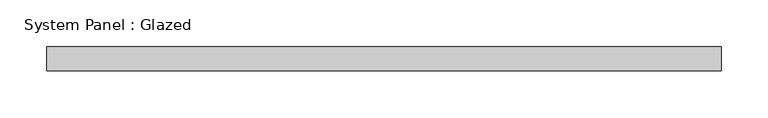
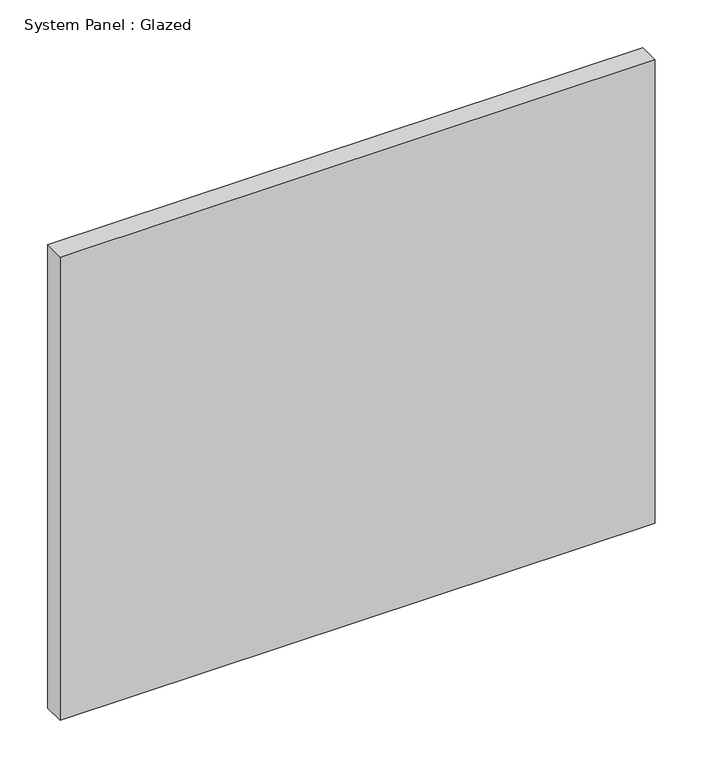
"""IFC4 building model written with IfcOpenShell, lengths in millimetres: plate geometry, System Panel : Glazed."""

from ifc_helpers import new_model, si_unit, origin, origin_with_axes, place, context, project, spatial, polyline, outline, extrude, source, transform, mapped, element, save


def system_panel_glazed_ba8d0b35(model_context):
    return source(origin(), model_context, "Body", "SweptSolid", [
        extrude(outline(polyline([(358.775, 19.05), (-358.775, 19.05), (-358.775, 44.45), (358.775, 44.45), (358.775, 19.05)])), origin_with_axes(), (0.0, 0.0, 1.0), 590.2074877),
    ])


if __name__ == "__main__":
    model = new_model("IFC4")
    model_context = context("Model", 3, world=origin())
    ifc_project = project(units=[si_unit("LENGTHUNIT", "METRE", prefix="MILLI")], contexts=[model_context])
    site = spatial("IfcSite", under=ifc_project)
    building = spatial("IfcBuilding", under=site)
    placement = place(None, origin())
    system_panel_glazed_shape = system_panel_glazed_ba8d0b35(model_context)
    element("IfcPlate", 1, ObjectType="System Panel : Glazed", at=placement, inside=building, context=model_context, shape_type="MappedRepresentation", body=[
        mapped(system_panel_glazed_shape, transform((0.0, 0.0, 0.0), x_axis=(1.0, 0.0, 0.0), y_axis=(0.0, 1.0, 0.0), z_axis=(0.0, 0.0, 1.0))),
    ])
    save(model, "model.ifc")

# Revit data of these elements
# Type "System Panel : Glazed"
#   Construction Type Id = "GSP4R"
#   Analytic Construction = "1/8 in Pilkington single glazing"
#   Visual Light Transmittance = 0.9
#   Solar Heat Gain Coefficient = 0.86
#   Heat Transfer Coefficient (U) = 1.18115 BTU/(h·ft²·°F)
#   Define Thermal Properties by = 1
# Element 1 (IfcPlate, "System Panel : Glazed")
#   Materials on its faces: "Glass"
# Materials
#   "Glass": class "Glass", colour RGB 0 128 192, transparency 0.75, Description = "Soda Lime Glass", Cost = 0
